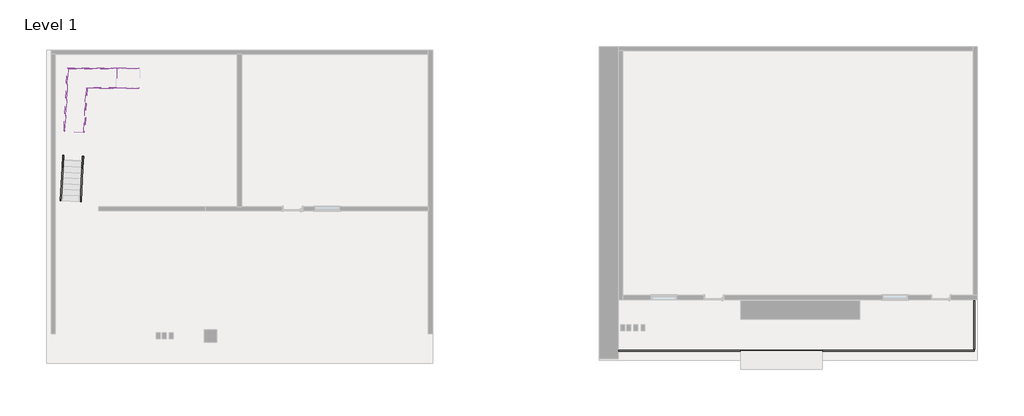
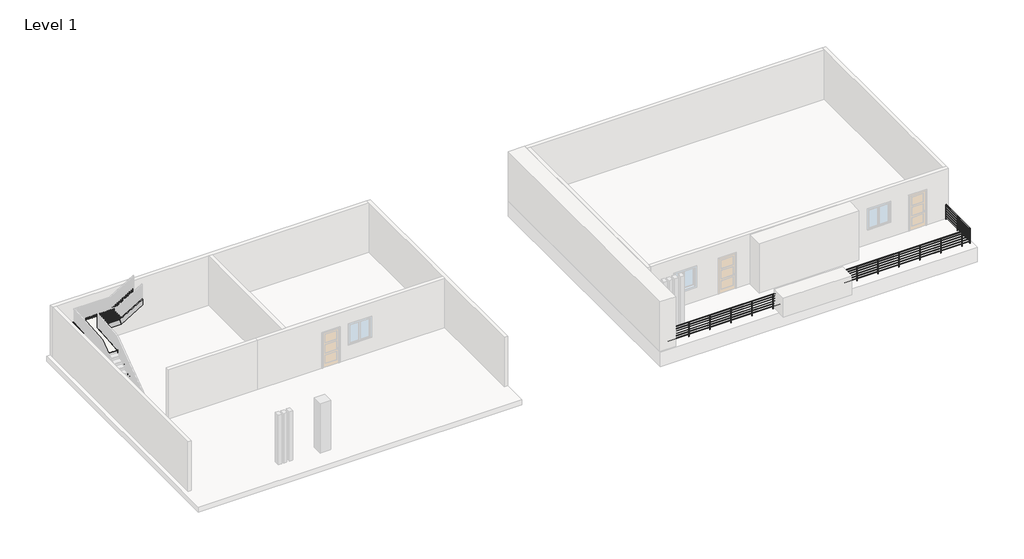
# One storey, part 3 of 3: 8 members, 2 railings, 1 slab.
"""IFC4 building model written with IfcOpenShell, lengths in millimetres."""

from ifc_helpers import new_model, si_unit, point, frame, frame_2d, origin, origin_with_axes, place, context, project, spatial, polyline, circle_curve, trimmed, segment, composite_curve, outline, extrude, faceted_brep, transform, mapped, element, save
from components import non_monolithic_landing_6dfc5b97

model = new_model("IFC4")

# Units and contexts
model_context = context("Model", 3, world=origin())
ifc_project = project(units=[si_unit("LENGTHUNIT", "METRE", prefix="MILLI")], contexts=[model_context])

# Site, building, storey
site = spatial("IfcSite", under=ifc_project)
building = spatial("IfcBuilding", under=site)
storey = spatial("IfcBuildingStorey", under=building, Name="Level 1", Elevation=0.0)

# Members
placement = place(None, origin())
element("IfcMember", 1, ObjectType="Stringer - 2\" Width", at=placement, inside=storey, context=model_context, shape_type="SweptSolid", body=[
    extrude(outline(polyline([(184.7272728, -304.8000001), (74.7879572, -123.4001294), (278.3981706, 0.0), (4084.5467363, 0.0), (4169.7011928, -304.8), (184.7272728, -304.8000001)])), frame((-19614.0949489, 10767.2493231, -144.2942496), z_axis=(-0.9986295347545739, 0.05233595624294519, 0.0), x_axis=(0.044757596291274584, 0.8540258126479454, 0.5183017160932845)), (0.0, 0.0, 1.0), 50.8),
])
element("IfcMember", 2, ObjectType="Stringer - 2\" Width", at=placement, inside=storey, context=model_context, shape_type="SweptSolid", body=[
    extrude(outline(polyline([(184.7272728, -304.8000001), (74.7879572, -123.4001294), (278.3981706, 0.0), (4084.5467363, 0.0), (4169.7011928, -304.8), (184.7272728, -304.8000001)])), frame((-18650.217722, 10716.7346581, -144.2942496), z_axis=(-0.9986295347545739, 0.052335956242945195, 0.0), x_axis=(0.044757596291274564, 0.854025812647945, 0.5183017160932853)), (0.0, 0.0, 1.0), 50.8),
])
element("IfcMember", 3, ObjectType="Stringer - 2\" Width", at=placement, inside=storey, context=model_context, shape_type="SweptSolid", body=[
    extrude(outline(polyline([(2277.5333333, -17174.5928737), (1972.7333333, -17089.4384172), (2734.3724171, -15832.733929), (3090.7811786, -15832.733929), (2277.5333333, -17174.5928737)])), frame((0.0, 17185.5159704, 0.0), z_axis=(0.0, 1.0, 0.0), x_axis=(0.0, 0.0, 1.0)), (0.0, 0.0, 1.0), 50.8),
])
element("IfcMember", 4, ObjectType="Stringer - 2\" Width", at=placement, inside=storey, context=model_context, shape_type="SweptSolid", body=[
    extrude(outline(polyline([(2277.5333333, -17174.5928737), (1972.7333333, -17089.4384172), (2734.3724171, -15832.733929), (3090.7811786, -15832.733929), (2277.5333333, -17174.5928737)])), frame((0.0, 16220.3159704, 0.0), z_axis=(0.0, 1.0, 0.0), x_axis=(0.0, 0.0, 1.0)), (0.0, 0.0, 1.0), 50.8),
])
element("IfcMember", 5, ObjectType="Stringer - 2\" Width", at=placement, inside=storey, context=model_context, shape_type="Brep", body=[
    faceted_brep([(-17174.5928737, 17185.5159704, 2277.5333333), (-17174.5928737, 17236.3159704, 2277.5333333), (-19325.9352471, 17236.3159704, 2277.5333333), (-19277.7278471, 17185.5159704, 2277.5333333), (-17089.4384172, 17185.5159704, 1972.7333333), (-19277.7278471, 17185.5159704, 1972.7333333), (-17089.4384172, 17236.3159704, 1972.7333333), (-19325.9352471, 17236.3159704, 1972.7333333)], [[[0, 1, 2, 3]], [[4, 0, 3, 5]], [[6, 4, 5, 7]], [[1, 6, 7, 2]], [[1, 0, 4, 6]], [[2, 7, 5, 3]]]),
])
element("IfcMember", 6, ObjectType="Stringer - 2\" Width", at=placement, inside=storey, context=model_context, shape_type="Brep", body=[
    faceted_brep([(-19277.7278471, 17185.5159704, 2277.5333333), (-19325.9352471, 17236.3159704, 2277.5333333), (-19486.4674753, 14173.1785802, 2277.5333333), (-19435.737095, 14170.5199136, 2277.5333333), (-19277.7278471, 17185.5159704, 1972.7333333), (-19431.2804551, 14255.5576689, 1972.7333333), (-19325.9352471, 17236.3159704, 1972.7333333), (-19482.0108354, 14258.2163355, 1972.7333333)], [[[0, 1, 2, 3]], [[4, 0, 3, 5]], [[6, 4, 5, 7]], [[1, 6, 7, 2]], [[1, 0, 4, 6]], [[2, 7, 5, 3]]]),
])
element("IfcMember", 7, ObjectType="Stringer - 2\" Width", at=placement, inside=storey, context=model_context, shape_type="Brep", body=[
    faceted_brep([(-18522.5902484, 14122.6639152, 2277.5333333), (-18471.859868, 14120.0052486, 2277.5333333), (-18361.7872473, 16220.3159704, 2277.5333333), (-18409.9946473, 16271.1159704, 2277.5333333), (-18518.1336085, 14207.7016705, 1972.7333333), (-18409.9946473, 16271.1159704, 1972.7333333), (-18467.4032281, 14205.0430039, 1972.7333333), (-18361.7872473, 16220.3159704, 1972.7333333)], [[[0, 1, 2, 3]], [[4, 0, 3, 5]], [[6, 4, 5, 7]], [[1, 6, 7, 2]], [[1, 0, 4, 6]], [[2, 7, 5, 3]]]),
])
element("IfcMember", 8, ObjectType="Stringer - 2\" Width", at=placement, inside=storey, context=model_context, shape_type="Brep", body=[
    faceted_brep([(-18409.9946473, 16271.1159704, 2277.5333333), (-18361.7872473, 16220.3159704, 2277.5333333), (-17174.5928737, 16220.3159704, 2277.5333333), (-17174.5928737, 16271.1159704, 2277.5333333), (-18409.9946473, 16271.1159704, 1972.7333333), (-17089.4384172, 16271.1159704, 1972.7333333), (-18361.7872473, 16220.3159704, 1972.7333333), (-17089.4384172, 16220.3159704, 1972.7333333)], [[[0, 1, 2, 3]], [[4, 0, 3, 5]], [[6, 4, 5, 7]], [[1, 6, 7, 2]], [[1, 0, 4, 6]], [[2, 7, 5, 3]]]),
])

# Railings
element("IfcRailing", 9, ObjectType="Handrail - Pipe", at=placement, inside=storey, context=model_context, shape_type="SweptSolid", body=[
    extrude(outline(composite_curve([segment(trimmed(circle_curve(frame_2d((3466.949368, 895.35)), 19.05), [point((3447.899368, 895.35))], [point((3485.999368, 895.35))], False, "CARTESIAN"), True, "CONTINUOUS"), segment(trimmed(circle_curve(frame_2d((3466.949368, 895.35)), 19.05), [point((3485.999368, 895.35))], [point((3447.899368, 895.35))], False, "CARTESIAN"), True, "CONTINUOUS")], self_intersect=False)), frame((7291.311019, 0.0, 0.0), z_axis=(1.0, 0.0, 0.0), x_axis=(0.0, 1.0, 0.0)), (0.0, 0.0, 1.0), 17551.4),
    extrude(outline(composite_curve([segment(trimmed(circle_curve(frame_2d((3466.949368, 749.3)), 12.7), [point((3479.649368, 749.3))], [point((3454.249368, 749.3))], False, "CARTESIAN"), True, "CONTINUOUS"), segment(trimmed(circle_curve(frame_2d((3466.949368, 749.3)), 12.7), [point((3454.249368, 749.3))], [point((3479.649368, 749.3))], False, "CARTESIAN"), True, "CONTINUOUS")], self_intersect=False)), frame((7291.311019, 0.0, 0.0), z_axis=(1.0, 0.0, 0.0), x_axis=(0.0, 1.0, 0.0)), (0.0, 0.0, 1.0), 17551.4),
    extrude(outline(composite_curve([segment(trimmed(circle_curve(frame_2d((3466.949368, 596.9)), 12.7), [point((3479.649368, 596.9))], [point((3454.249368, 596.9))], False, "CARTESIAN"), True, "CONTINUOUS"), segment(trimmed(circle_curve(frame_2d((3466.949368, 596.9)), 12.7), [point((3454.249368, 596.9))], [point((3479.649368, 596.9))], False, "CARTESIAN"), True, "CONTINUOUS")], self_intersect=False)), frame((7291.311019, 0.0, 0.0), z_axis=(1.0, 0.0, 0.0), x_axis=(0.0, 1.0, 0.0)), (0.0, 0.0, 1.0), 17551.4),
    extrude(outline(composite_curve([segment(trimmed(circle_curve(frame_2d((3466.949368, 444.5)), 12.7), [point((3479.649368, 444.5))], [point((3454.249368, 444.5))], False, "CARTESIAN"), True, "CONTINUOUS"), segment(trimmed(circle_curve(frame_2d((3466.949368, 444.5)), 12.7), [point((3454.249368, 444.5))], [point((3479.649368, 444.5))], False, "CARTESIAN"), True, "CONTINUOUS")], self_intersect=False)), frame((7291.311019, 0.0, 0.0), z_axis=(1.0, 0.0, 0.0), x_axis=(0.0, 1.0, 0.0)), (0.0, 0.0, 1.0), 17551.4),
    extrude(outline(composite_curve([segment(trimmed(circle_curve(frame_2d((3466.949368, 292.1)), 12.7), [point((3479.649368, 292.1))], [point((3454.249368, 292.1))], False, "CARTESIAN"), True, "CONTINUOUS"), segment(trimmed(circle_curve(frame_2d((3466.949368, 292.1)), 12.7), [point((3454.249368, 292.1))], [point((3479.649368, 292.1))], False, "CARTESIAN"), True, "CONTINUOUS")], self_intersect=False)), frame((7291.311019, 0.0, 0.0), z_axis=(1.0, 0.0, 0.0), x_axis=(0.0, 1.0, 0.0)), (0.0, 0.0, 1.0), 17551.4),
    extrude(outline(composite_curve([segment(trimmed(circle_curve(frame_2d((3466.949368, 139.7)), 12.7), [point((3479.649368, 139.7))], [point((3454.249368, 139.7))], False, "CARTESIAN"), True, "CONTINUOUS"), segment(trimmed(circle_curve(frame_2d((3466.949368, 139.7)), 12.7), [point((3454.249368, 139.7))], [point((3479.649368, 139.7))], False, "CARTESIAN"), True, "CONTINUOUS")], self_intersect=False)), frame((7291.311019, 0.0, 0.0), z_axis=(1.0, 0.0, 0.0), x_axis=(0.0, 1.0, 0.0)), (0.0, 0.0, 1.0), 17551.4),
    extrude(outline(composite_curve([segment(trimmed(circle_curve(frame_2d((24360.111019, 3466.949368)), 12.7), [point((24360.111019, 3479.649368))], [point((24360.111019, 3454.249368))], False, "CARTESIAN"), True, "CONTINUOUS"), segment(trimmed(circle_curve(frame_2d((24360.111019, 3466.949368)), 12.7), [point((24360.111019, 3454.249368))], [point((24360.111019, 3479.649368))], False, "CARTESIAN"), True, "CONTINUOUS")], self_intersect=False)), origin_with_axes(), (0.0, 0.0, 1.0), 876.3),
    extrude(outline(composite_curve([segment(trimmed(circle_curve(frame_2d((23140.911019, 3466.949368)), 12.7), [point((23140.911019, 3479.649368))], [point((23140.911019, 3454.249368))], False, "CARTESIAN"), True, "CONTINUOUS"), segment(trimmed(circle_curve(frame_2d((23140.911019, 3466.949368)), 12.7), [point((23140.911019, 3454.249368))], [point((23140.911019, 3479.649368))], False, "CARTESIAN"), True, "CONTINUOUS")], self_intersect=False)), origin_with_axes(), (0.0, 0.0, 1.0), 876.3),
    extrude(outline(composite_curve([segment(trimmed(circle_curve(frame_2d((21921.711019, 3466.949368)), 12.7), [point((21921.711019, 3479.649368))], [point((21921.711019, 3454.249368))], False, "CARTESIAN"), True, "CONTINUOUS"), segment(trimmed(circle_curve(frame_2d((21921.711019, 3466.949368)), 12.7), [point((21921.711019, 3454.249368))], [point((21921.711019, 3479.649368))], False, "CARTESIAN"), True, "CONTINUOUS")], self_intersect=False)), origin_with_axes(), (0.0, 0.0, 1.0), 876.3),
    extrude(outline(composite_curve([segment(trimmed(circle_curve(frame_2d((20702.511019, 3466.949368)), 12.7), [point((20702.511019, 3479.649368))], [point((20702.511019, 3454.249368))], False, "CARTESIAN"), True, "CONTINUOUS"), segment(trimmed(circle_curve(frame_2d((20702.511019, 3466.949368)), 12.7), [point((20702.511019, 3454.249368))], [point((20702.511019, 3479.649368))], False, "CARTESIAN"), True, "CONTINUOUS")], self_intersect=False)), origin_with_axes(), (0.0, 0.0, 1.0), 876.3),
    extrude(outline(composite_curve([segment(trimmed(circle_curve(frame_2d((19483.311019, 3466.949368)), 12.7), [point((19483.311019, 3479.649368))], [point((19483.311019, 3454.249368))], False, "CARTESIAN"), True, "CONTINUOUS"), segment(trimmed(circle_curve(frame_2d((19483.311019, 3466.949368)), 12.7), [point((19483.311019, 3454.249368))], [point((19483.311019, 3479.649368))], False, "CARTESIAN"), True, "CONTINUOUS")], self_intersect=False)), origin_with_axes(), (0.0, 0.0, 1.0), 876.3),
    extrude(outline(composite_curve([segment(trimmed(circle_curve(frame_2d((18264.111019, 3466.949368)), 12.7), [point((18264.111019, 3479.649368))], [point((18264.111019, 3454.249368))], False, "CARTESIAN"), True, "CONTINUOUS"), segment(trimmed(circle_curve(frame_2d((18264.111019, 3466.949368)), 12.7), [point((18264.111019, 3454.249368))], [point((18264.111019, 3479.649368))], False, "CARTESIAN"), True, "CONTINUOUS")], self_intersect=False)), origin_with_axes(), (0.0, 0.0, 1.0), 876.3),
    extrude(outline(composite_curve([segment(trimmed(circle_curve(frame_2d((17044.911019, 3466.949368)), 12.7), [point((17044.911019, 3479.649368))], [point((17044.911019, 3454.249368))], False, "CARTESIAN"), True, "CONTINUOUS"), segment(trimmed(circle_curve(frame_2d((17044.911019, 3466.949368)), 12.7), [point((17044.911019, 3454.249368))], [point((17044.911019, 3479.649368))], False, "CARTESIAN"), True, "CONTINUOUS")], self_intersect=False)), origin_with_axes(), (0.0, 0.0, 1.0), 876.3),
    extrude(outline(composite_curve([segment(trimmed(circle_curve(frame_2d((15825.711019, 3466.949368)), 12.7), [point((15825.711019, 3479.649368))], [point((15825.711019, 3454.249368))], False, "CARTESIAN"), True, "CONTINUOUS"), segment(trimmed(circle_curve(frame_2d((15825.711019, 3466.949368)), 12.7), [point((15825.711019, 3454.249368))], [point((15825.711019, 3479.649368))], False, "CARTESIAN"), True, "CONTINUOUS")], self_intersect=False)), origin_with_axes(), (0.0, 0.0, 1.0), 876.3),
    extrude(outline(composite_curve([segment(trimmed(circle_curve(frame_2d((14606.511019, 3466.949368)), 12.7), [point((14606.511019, 3479.649368))], [point((14606.511019, 3454.249368))], False, "CARTESIAN"), True, "CONTINUOUS"), segment(trimmed(circle_curve(frame_2d((14606.511019, 3466.949368)), 12.7), [point((14606.511019, 3454.249368))], [point((14606.511019, 3479.649368))], False, "CARTESIAN"), True, "CONTINUOUS")], self_intersect=False)), origin_with_axes(), (0.0, 0.0, 1.0), 876.3),
    extrude(outline(composite_curve([segment(trimmed(circle_curve(frame_2d((13387.311019, 3466.949368)), 12.7), [point((13387.311019, 3479.649368))], [point((13387.311019, 3454.249368))], False, "CARTESIAN"), True, "CONTINUOUS"), segment(trimmed(circle_curve(frame_2d((13387.311019, 3466.949368)), 12.7), [point((13387.311019, 3454.249368))], [point((13387.311019, 3479.649368))], False, "CARTESIAN"), True, "CONTINUOUS")], self_intersect=False)), origin_with_axes(), (0.0, 0.0, 1.0), 876.3),
    extrude(outline(composite_curve([segment(trimmed(circle_curve(frame_2d((12168.111019, 3466.949368)), 12.7), [point((12168.111019, 3479.649368))], [point((12168.111019, 3454.249368))], False, "CARTESIAN"), True, "CONTINUOUS"), segment(trimmed(circle_curve(frame_2d((12168.111019, 3466.949368)), 12.7), [point((12168.111019, 3454.249368))], [point((12168.111019, 3479.649368))], False, "CARTESIAN"), True, "CONTINUOUS")], self_intersect=False)), origin_with_axes(), (0.0, 0.0, 1.0), 876.3),
    extrude(outline(composite_curve([segment(trimmed(circle_curve(frame_2d((10948.911019, 3466.949368)), 12.7), [point((10948.911019, 3479.649368))], [point((10948.911019, 3454.249368))], False, "CARTESIAN"), True, "CONTINUOUS"), segment(trimmed(circle_curve(frame_2d((10948.911019, 3466.949368)), 12.7), [point((10948.911019, 3454.249368))], [point((10948.911019, 3479.649368))], False, "CARTESIAN"), True, "CONTINUOUS")], self_intersect=False)), origin_with_axes(), (0.0, 0.0, 1.0), 876.3),
    extrude(outline(composite_curve([segment(trimmed(circle_curve(frame_2d((9729.711019, 3466.949368)), 12.7), [point((9729.711019, 3479.649368))], [point((9729.711019, 3454.249368))], False, "CARTESIAN"), True, "CONTINUOUS"), segment(trimmed(circle_curve(frame_2d((9729.711019, 3466.949368)), 12.7), [point((9729.711019, 3454.249368))], [point((9729.711019, 3479.649368))], False, "CARTESIAN"), True, "CONTINUOUS")], self_intersect=False)), origin_with_axes(), (0.0, 0.0, 1.0), 876.3),
    extrude(outline(composite_curve([segment(trimmed(circle_curve(frame_2d((8510.511019, 3466.949368)), 12.7), [point((8510.511019, 3479.649368))], [point((8510.511019, 3454.249368))], False, "CARTESIAN"), True, "CONTINUOUS"), segment(trimmed(circle_curve(frame_2d((8510.511019, 3466.949368)), 12.7), [point((8510.511019, 3454.249368))], [point((8510.511019, 3479.649368))], False, "CARTESIAN"), True, "CONTINUOUS")], self_intersect=False)), origin_with_axes(), (0.0, 0.0, 1.0), 876.3),
    extrude(outline(composite_curve([segment(trimmed(circle_curve(frame_2d((24830.011019, 3466.949368)), 12.7), [point((24830.011019, 3479.649368))], [point((24830.011019, 3454.249368))], False, "CARTESIAN"), True, "CONTINUOUS"), segment(trimmed(circle_curve(frame_2d((24830.011019, 3466.949368)), 12.7), [point((24830.011019, 3454.249368))], [point((24830.011019, 3479.649368))], False, "CARTESIAN"), True, "CONTINUOUS")], self_intersect=False)), origin_with_axes(), (0.0, 0.0, 1.0), 876.3),
    extrude(outline(composite_curve([segment(trimmed(circle_curve(frame_2d((7304.011019, 3466.949368)), 12.7), [point((7304.011019, 3479.649368))], [point((7304.011019, 3454.249368))], False, "CARTESIAN"), True, "CONTINUOUS"), segment(trimmed(circle_curve(frame_2d((7304.011019, 3466.949368)), 12.7), [point((7304.011019, 3454.249368))], [point((7304.011019, 3479.649368))], False, "CARTESIAN"), True, "CONTINUOUS")], self_intersect=False)), origin_with_axes(), (0.0, 0.0, 1.0), 876.3),
])
element("IfcRailing", 10, ObjectType="Handrail - Pipe", at=placement, inside=storey, context=model_context, shape_type="SweptSolid", body=[
    extrude(outline(composite_curve([segment(trimmed(circle_curve(frame_2d((895.35, 24842.711019)), 19.05), [point((895.35, 24861.761019))], [point((895.35, 24823.661019))], False, "CARTESIAN"), True, "CONTINUOUS"), segment(trimmed(circle_curve(frame_2d((895.35, 24842.711019)), 19.05), [point((895.35, 24823.661019))], [point((895.35, 24861.761019))], False, "CARTESIAN"), True, "CONTINUOUS")], self_intersect=False)), frame((0.0, 3543.149368, 0.0), z_axis=(0.0, 1.0, 0.0), x_axis=(0.0, 0.0, 1.0)), (0.0, 0.0, 1.0), 2362.2),
    extrude(outline(composite_curve([segment(trimmed(circle_curve(frame_2d((749.3, 24842.711019)), 12.7), [point((749.3, 24830.011019))], [point((749.3, 24855.411019))], False, "CARTESIAN"), True, "CONTINUOUS"), segment(trimmed(circle_curve(frame_2d((749.3, 24842.711019)), 12.7), [point((749.3, 24855.411019))], [point((749.3, 24830.011019))], False, "CARTESIAN"), True, "CONTINUOUS")], self_intersect=False)), frame((0.0, 3543.149368, 0.0), z_axis=(0.0, 1.0, 0.0), x_axis=(0.0, 0.0, 1.0)), (0.0, 0.0, 1.0), 2362.2),
    extrude(outline(composite_curve([segment(trimmed(circle_curve(frame_2d((596.9, 24842.711019)), 12.7), [point((596.9, 24830.011019))], [point((596.9, 24855.411019))], False, "CARTESIAN"), True, "CONTINUOUS"), segment(trimmed(circle_curve(frame_2d((596.9, 24842.711019)), 12.7), [point((596.9, 24855.411019))], [point((596.9, 24830.011019))], False, "CARTESIAN"), True, "CONTINUOUS")], self_intersect=False)), frame((0.0, 3543.149368, 0.0), z_axis=(0.0, 1.0, 0.0), x_axis=(0.0, 0.0, 1.0)), (0.0, 0.0, 1.0), 2362.2),
    extrude(outline(composite_curve([segment(trimmed(circle_curve(frame_2d((444.5, 24842.711019)), 12.7), [point((444.5, 24830.011019))], [point((444.5, 24855.411019))], False, "CARTESIAN"), True, "CONTINUOUS"), segment(trimmed(circle_curve(frame_2d((444.5, 24842.711019)), 12.7), [point((444.5, 24855.411019))], [point((444.5, 24830.011019))], False, "CARTESIAN"), True, "CONTINUOUS")], self_intersect=False)), frame((0.0, 3543.149368, 0.0), z_axis=(0.0, 1.0, 0.0), x_axis=(0.0, 0.0, 1.0)), (0.0, 0.0, 1.0), 2362.2),
    extrude(outline(composite_curve([segment(trimmed(circle_curve(frame_2d((292.1, 24842.711019)), 12.7), [point((292.1, 24830.011019))], [point((292.1, 24855.411019))], False, "CARTESIAN"), True, "CONTINUOUS"), segment(trimmed(circle_curve(frame_2d((292.1, 24842.711019)), 12.7), [point((292.1, 24855.411019))], [point((292.1, 24830.011019))], False, "CARTESIAN"), True, "CONTINUOUS")], self_intersect=False)), frame((0.0, 3543.149368, 0.0), z_axis=(0.0, 1.0, 0.0), x_axis=(0.0, 0.0, 1.0)), (0.0, 0.0, 1.0), 2362.2),
    extrude(outline(composite_curve([segment(trimmed(circle_curve(frame_2d((139.7, 24842.711019)), 12.7), [point((139.7, 24830.011019))], [point((139.7, 24855.411019))], False, "CARTESIAN"), True, "CONTINUOUS"), segment(trimmed(circle_curve(frame_2d((139.7, 24842.711019)), 12.7), [point((139.7, 24855.411019))], [point((139.7, 24830.011019))], False, "CARTESIAN"), True, "CONTINUOUS")], self_intersect=False)), frame((0.0, 3543.149368, 0.0), z_axis=(0.0, 1.0, 0.0), x_axis=(0.0, 0.0, 1.0)), (0.0, 0.0, 1.0), 2362.2),
    extrude(outline(composite_curve([segment(trimmed(circle_curve(frame_2d((24842.711019, 4762.349368)), 12.7), [point((24830.011019, 4762.349368))], [point((24855.411019, 4762.349368))], False, "CARTESIAN"), True, "CONTINUOUS"), segment(trimmed(circle_curve(frame_2d((24842.711019, 4762.349368)), 12.7), [point((24855.411019, 4762.349368))], [point((24830.011019, 4762.349368))], False, "CARTESIAN"), True, "CONTINUOUS")], self_intersect=False)), origin_with_axes(), (0.0, 0.0, 1.0), 876.3),
    extrude(outline(composite_curve([segment(trimmed(circle_curve(frame_2d((24842.711019, 5892.649368)), 12.7), [point((24830.011019, 5892.649368))], [point((24855.411019, 5892.649368))], False, "CARTESIAN"), True, "CONTINUOUS"), segment(trimmed(circle_curve(frame_2d((24842.711019, 5892.649368)), 12.7), [point((24855.411019, 5892.649368))], [point((24830.011019, 5892.649368))], False, "CARTESIAN"), True, "CONTINUOUS")], self_intersect=False)), origin_with_axes(), (0.0, 0.0, 1.0), 876.3),
    extrude(outline(composite_curve([segment(trimmed(circle_curve(frame_2d((24842.711019, 3555.849368)), 12.7), [point((24830.011019, 3555.849368))], [point((24855.411019, 3555.849368))], False, "CARTESIAN"), True, "CONTINUOUS"), segment(trimmed(circle_curve(frame_2d((24842.711019, 3555.849368)), 12.7), [point((24855.411019, 3555.849368))], [point((24830.011019, 3555.849368))], False, "CARTESIAN"), True, "CONTINUOUS")], self_intersect=False)), origin_with_axes(), (0.0, 0.0, 1.0), 876.3),
])

# Slab
non_monolithic_landing_shape = non_monolithic_landing_6dfc5b97(model_context)
element("IfcSlab", 11, ObjectType="Non-Monolithic Landing", at=placement, inside=storey, context=model_context, shape_type="MappedRepresentation", body=[
    mapped(non_monolithic_landing_shape, transform((0.0, 0.0, 0.0), x_axis=(1.0, 0.0, 0.0), y_axis=(0.0, 1.0, 0.0), z_axis=(0.0, 0.0, 1.0))),
])

save(model, "model.ifc")

# Revit data of these elements
# Type "Handrail - Pipe"
#   Assembly Code = "C2010400"
#   built-in parameter 1008612 = 0.0416667 (stored number, unit not read)
#   built-in parameter 1008611 = 0.0833333 (stored number, unit not read)
#   built-in parameter 1008609 = 4 (stored number, unit not read)
#   built-in parameter 1008604 = 0.166667 (stored number, unit not read)
#   built-in parameter 1008603 = 0.166667 (stored number, unit not read)
#   Railing Height = 3' - 0"
#   built-in parameter 1008630 = 2
#   built-in parameter 1008610 = 1
#   built-in parameter 1008605 = 1
#   built-in parameter 1008618 = Baluster - Round : 1"
# Elements 1, 2, 3, 4, 5, 6, 7, 8 (IfcMember, "Stringer - 2\" Width")
#   Phase Created = New Construction
# Elements 9, 10 (IfcRailing, "Handrail - Pipe")
#   Phase Created = New Construction
# Element 11 (IfcSlab, "Non-Monolithic Landing")
#   Phase Created = New Construction
